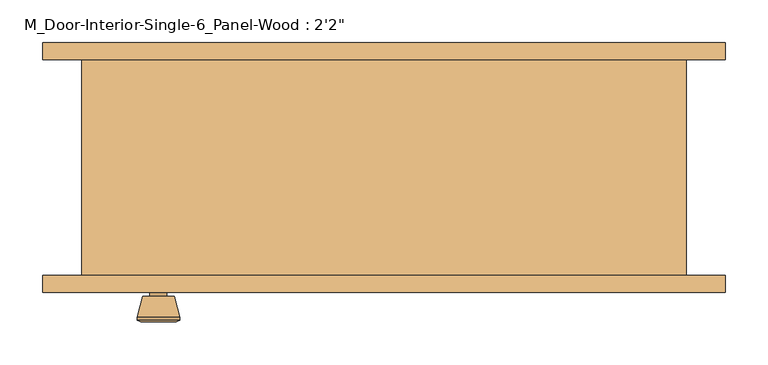
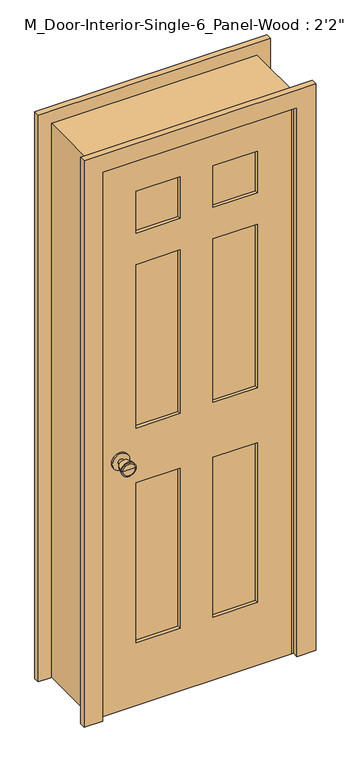
"""IFC4 building model written with IfcOpenShell, lengths in millimetres: door geometry."""

from ifc_helpers import new_model, si_unit, point, frame, frame_2d, origin, place, context, project, spatial, polyline, circle_curve, trimmed, segment, composite_curve, outline, extrude, faceted_brep, source, transform, mapped, element, save
from ifc_brep_helpers import plane_surface, cylinder_surface, revolved_surface, advanced_brep


def door_809e0d7a(model_context):
    return source(origin(), model_context, "Body", "SolidModel", [
        advanced_brep(
        [(-265.2, -82.825, 914.4), (-275.2, -82.825, 914.4), (-255.2, -82.825, 914.4), (-244.7241324, -33.825, 914.4), (-285.6758676, -33.825, 914.4), (-265.2, -33.825, 914.4), (-240.2, -35.6528681, 914.4), (-290.2, -35.6528681, 914.4), (-240.2, -39.1165463, 914.4), (-290.2, -39.1165463, 914.4), (-246.563764, -63.825, 914.4), (-283.836236, -63.825, 914.4), (-255.2, -63.825, 914.4), (-275.2, -63.825, 914.4)],
        [
            (0, 1),
            (1, 2, circle_curve(frame((-265.2, -82.825, 914.4), z_axis=(0.0, -1.0, 0.0), x_axis=(-1.0, 0.0, 0.0)), 10.0)),
            (2, 0),
            (2, 1, circle_curve(frame((-265.2, -82.825, 914.4), z_axis=(0.0, -1.0, 0.0), x_axis=(-1.0, 0.0, 0.0)), 10.0)),
            (3, 4, circle_curve(frame((-265.2, -33.825, 914.4), z_axis=(0.0, 1.0, 0.0), x_axis=(-1.0, 0.0, 0.0)), 20.4758676)),
            (4, 5),
            (5, 3),
            (4, 3, circle_curve(frame((-265.2, -33.825, 914.4), z_axis=(0.0, 1.0, 0.0), x_axis=(-1.0, 0.0, 0.0)), 20.4758676)),
            (6, 7, circle_curve(frame((-265.2, -35.6528681, 914.4), z_axis=(0.0, 1.0, 0.0), x_axis=(-1.0, 0.0, 0.0)), 25.0)),
            (7, 4),
            (3, 6),
            (7, 6, circle_curve(frame((-265.2, -35.6528681, 914.4), z_axis=(0.0, 1.0, 0.0), x_axis=(-1.0, 0.0, 0.0)), 25.0)),
            (8, 9, circle_curve(frame((-265.2, -39.1165463, 914.4), z_axis=(0.0, 1.0, 0.0), x_axis=(-1.0, 0.0, 0.0)), 25.0)),
            (9, 7),
            (6, 8),
            (9, 8, circle_curve(frame((-265.2, -39.1165463, 914.4), z_axis=(0.0, 1.0, 0.0), x_axis=(-1.0, 0.0, 0.0)), 25.0)),
            (10, 11, circle_curve(frame((-265.2, -63.825, 914.4), z_axis=(0.0, 1.0, 0.0), x_axis=(-1.0, 0.0, 0.0)), 18.636236)),
            (11, 9),
            (8, 10),
            (11, 10, circle_curve(frame((-265.2, -63.825, 914.4), z_axis=(0.0, 1.0, 0.0), x_axis=(-1.0, 0.0, 0.0)), 18.636236)),
            (12, 13, circle_curve(frame((-265.2, -63.825, 914.4), z_axis=(0.0, 1.0, 0.0), x_axis=(-1.0, 0.0, 0.0)), 10.0)),
            (13, 11),
            (10, 12),
            (13, 12, circle_curve(frame((-265.2, -63.825, 914.4), z_axis=(0.0, 1.0, 0.0), x_axis=(-1.0, 0.0, 0.0)), 10.0)),
            (1, 13),
            (12, 2),
        ],
        [
            plane_surface(frame((-265.2, -82.825, 914.4), z_axis=(0.0, -1.0, 0.0), x_axis=(-1.0, 0.0, 0.0))),
            plane_surface(frame((-265.2, -33.825, 914.4), z_axis=(0.0, 1.0, 0.0), x_axis=(-1.0, 0.0, 0.0))),
            revolved_surface(polyline([(-285.6758676, -33.825, 914.4), (-290.2, -35.6528681, 914.4)]), (-265.2, -82.825, 914.4), (0.0, -1.0, 0.0)),
            cylinder_surface(frame((-265.2, -82.825, 914.4), z_axis=(0.0, -1.0, 0.0), x_axis=(-1.0, 0.0, 0.0)), 25.0),
            revolved_surface(polyline([(-290.2, -39.1165463, 914.4), (-283.836236, -63.825, 914.4)]), (-265.2, -82.825, 914.4), (0.0, -1.0, 0.0)),
            plane_surface(frame((-265.2, -63.825, 914.4), z_axis=(0.0, -1.0, 0.0), x_axis=(-1.0, 0.0, 0.0))),
            cylinder_surface(frame((-265.2, -82.825, 914.4), z_axis=(0.0, -1.0, 0.0), x_axis=(-1.0, 0.0, 0.0)), 10.0),
        ],
        [
            (0, [[1, 2, 3]]),
            (0, [[-3, 4, -1]]),
            (1, [[5, 6, 7]]),
            (1, [[8, -7, -6]]),
            (2, [[9, 10, -5, 11]]),
            (2, [[12, -11, -8, -10]]),
            (3, [[13, 14, -9, 15]]),
            (3, [[16, -15, -12, -14]]),
            (4, [[17, 18, -13, 19]]),
            (4, [[20, -19, -16, -18]]),
            (5, [[21, 22, -17, 23]]),
            (5, [[24, -23, -20, -22]]),
            (6, [[-2, 25, -21, 26]]),
            (6, [[-4, -26, -24, -25]]),
        ],
    ),
        extrude(outline(composite_curve([segment(trimmed(circle_curve(frame_2d((914.4, -265.2)), 30.0), [point((914.4, -295.2))], [point((914.4, -235.2))], False, "CARTESIAN"), True, "CONTINUOUS"), segment(trimmed(circle_curve(frame_2d((914.4, -265.2)), 30.0), [point((914.4, -235.2))], [point((914.4, -295.2))], False, "CARTESIAN"), True, "CONTINUOUS")], self_intersect=False)), frame((0.0, -88.825, 0.0), z_axis=(0.0, 1.0, 0.0), x_axis=(0.0, 0.0, 1.0)), (0.0, 0.0, 1.0), 6.0),
        advanced_brep(
        [(-265.2, -129.825, 914.4), (-255.2, -129.825, 914.4), (-275.2, -129.825, 914.4), (-244.7241324, -178.825, 914.4), (-265.2, -178.825, 914.4), (-285.6758676, -178.825, 914.4), (-240.2, -176.9971319, 914.4), (-290.2, -176.9971319, 914.4), (-240.2, -173.5334537, 914.4), (-290.2, -173.5334537, 914.4), (-246.563764, -148.825, 914.4), (-283.836236, -148.825, 914.4), (-255.2, -148.825, 914.4), (-275.2, -148.825, 914.4)],
        [
            (0, 1),
            (1, 2, circle_curve(frame((-265.2, -129.825, 914.4), z_axis=(0.0, 1.0, 0.0), x_axis=(-1.0, 0.0, 0.0)), 10.0)),
            (2, 0),
            (2, 1, circle_curve(frame((-265.2, -129.825, 914.4), z_axis=(0.0, 1.0, 0.0), x_axis=(-1.0, 0.0, 0.0)), 10.0)),
            (3, 4),
            (4, 5),
            (5, 3, circle_curve(frame((-265.2, -178.825, 914.4), z_axis=(0.0, -1.0, 0.0), x_axis=(-1.0, 0.0, 0.0)), 20.4758676)),
            (3, 5, circle_curve(frame((-265.2, -178.825, 914.4), z_axis=(0.0, -1.0, 0.0), x_axis=(-1.0, 0.0, 0.0)), 20.4758676)),
            (6, 3),
            (5, 7),
            (7, 6, circle_curve(frame((-265.2, -176.9971319, 914.4), z_axis=(0.0, -1.0, 0.0), x_axis=(-1.0, 0.0, 0.0)), 25.0)),
            (6, 7, circle_curve(frame((-265.2, -176.9971319, 914.4), z_axis=(0.0, -1.0, 0.0), x_axis=(-1.0, 0.0, 0.0)), 25.0)),
            (8, 6),
            (7, 9),
            (9, 8, circle_curve(frame((-265.2, -173.5334537, 914.4), z_axis=(0.0, -1.0, 0.0), x_axis=(-1.0, 0.0, 0.0)), 25.0)),
            (8, 9, circle_curve(frame((-265.2, -173.5334537, 914.4), z_axis=(0.0, -1.0, 0.0), x_axis=(-1.0, 0.0, 0.0)), 25.0)),
            (10, 8),
            (9, 11),
            (11, 10, circle_curve(frame((-265.2, -148.825, 914.4), z_axis=(0.0, -1.0, 0.0), x_axis=(-1.0, 0.0, 0.0)), 18.636236)),
            (10, 11, circle_curve(frame((-265.2, -148.825, 914.4), z_axis=(0.0, -1.0, 0.0), x_axis=(-1.0, 0.0, 0.0)), 18.636236)),
            (12, 10),
            (11, 13),
            (13, 12, circle_curve(frame((-265.2, -148.825, 914.4), z_axis=(0.0, -1.0, 0.0), x_axis=(-1.0, 0.0, 0.0)), 10.0)),
            (12, 13, circle_curve(frame((-265.2, -148.825, 914.4), z_axis=(0.0, -1.0, 0.0), x_axis=(-1.0, 0.0, 0.0)), 10.0)),
            (1, 12),
            (13, 2),
        ],
        [
            plane_surface(frame((-265.2, -129.825, 914.4), z_axis=(0.0, 1.0, 0.0), x_axis=(-1.0, 0.0, 0.0))),
            plane_surface(frame((-265.2, -178.825, 914.4), z_axis=(0.0, -1.0, 0.0), x_axis=(-1.0, 0.0, 0.0))),
            revolved_surface(polyline([(-285.6758676, -178.825, 914.4), (-290.2, -176.9971319, 914.4)]), (-265.2, -129.825, 914.4), (0.0, 1.0, 0.0)),
            cylinder_surface(frame((-265.2, -129.825, 914.4), z_axis=(0.0, 1.0, 0.0), x_axis=(-1.0, 0.0, 0.0)), 25.0),
            revolved_surface(polyline([(-290.2, -173.5334537, 914.4), (-283.836236, -148.825, 914.4)]), (-265.2, -129.825, 914.4), (0.0, 1.0, 0.0)),
            plane_surface(frame((-265.2, -148.825, 914.4), z_axis=(0.0, 1.0, 0.0), x_axis=(-1.0, 0.0, 0.0))),
            cylinder_surface(frame((-265.2, -129.825, 914.4), z_axis=(0.0, 1.0, 0.0), x_axis=(-1.0, 0.0, 0.0)), 10.0),
        ],
        [
            (0, [[1, 2, 3]]),
            (0, [[-3, 4, -1]]),
            (1, [[5, 6, 7]]),
            (1, [[-6, -5, 8]]),
            (2, [[9, -7, 10, 11]]),
            (2, [[-10, -8, -9, 12]]),
            (3, [[13, -11, 14, 15]]),
            (3, [[-14, -12, -13, 16]]),
            (4, [[17, -15, 18, 19]]),
            (4, [[-18, -16, -17, 20]]),
            (5, [[21, -19, 22, 23]]),
            (5, [[-22, -20, -21, 24]]),
            (6, [[25, -23, 26, -2]]),
            (6, [[-26, -24, -25, -4]]),
        ],
    ),
        extrude(outline(composite_curve([segment(trimmed(circle_curve(frame_2d((914.4, -265.2)), 30.0), [point((914.4, -295.2))], [point((914.4, -235.2))], False, "CARTESIAN"), True, "CONTINUOUS"), segment(trimmed(circle_curve(frame_2d((914.4, -265.2)), 30.0), [point((914.4, -235.2))], [point((914.4, -295.2))], False, "CARTESIAN"), True, "CONTINUOUS")], self_intersect=False)), frame((0.0, -129.825, 0.0), z_axis=(0.0, 1.0, 0.0), x_axis=(0.0, 0.0, 1.0)), (0.0, 0.0, 1.0), 6.0),
        faceted_brep([(355.2, -123.825, 0.0), (330.2, -123.825, 0.0), (330.2, -88.825, 0.0), (317.5, -88.825, 0.0), (317.5, -53.9, 0.0), (330.2, -53.9, 0.0), (330.2, 130.175, 0.0), (355.2, 130.175, 0.0), (355.2, 130.175, 2025.0), (355.2, -123.825, 2025.0), (330.2, 130.175, 2000.0), (-330.2, 130.175, 2000.0), (-330.2, 130.175, 0.0), (-355.2, 130.175, 0.0), (-355.2, 130.175, 2025.0), (330.2, -53.9, 2000.0), (317.5, -53.9, 1987.3), (-317.5, -53.9, 1987.3), (-317.5, -53.9, 0.0), (-330.2, -53.9, 0.0), (-330.2, -53.9, 2000.0), (317.5, -88.825, 1987.3), (330.2, -88.825, 2000.0), (-330.2, -88.825, 2000.0), (-330.2, -88.825, 0.0), (-317.5, -88.825, 0.0), (-317.5, -88.825, 1987.3), (330.2, -123.825, 2000.0), (-355.2, -123.825, 2025.0), (-355.2, -123.825, 0.0), (-330.2, -123.825, 0.0), (-330.2, -123.825, 2000.0)], [[[0, 1, 2, 3, 4, 5, 6, 7]], [[7, 8, 9, 0]], [[6, 10, 11, 12, 13, 14, 8, 7]], [[5, 15, 10, 6]], [[4, 16, 17, 18, 19, 20, 15, 5]], [[3, 21, 16, 4]], [[2, 22, 23, 24, 25, 26, 21, 3]], [[1, 27, 22, 2]], [[0, 9, 28, 29, 30, 31, 27, 1]], [[8, 14, 28, 9]], [[15, 20, 11, 10]], [[21, 26, 17, 16]], [[27, 31, 23, 22]], [[29, 13, 12, 19, 18, 25, 24, 30]], [[14, 13, 29, 28]], [[20, 19, 12, 11]], [[26, 25, 18, 17]], [[31, 30, 24, 23]]]),
        extrude(outline(polyline([(2000.0, -330.2), (0.0, -330.2), (0.0, 330.2), (2000.0, 330.2), (2000.0, -330.2)]), holes=[polyline([(1880.0, 57.5), (1880.0, 210.2), (1727.3, 210.2), (1727.3, 57.5), (1880.0, 57.5)]), polyline([(1612.3, 210.2), (1014.4, 210.2), (1014.4, 57.5), (1612.3, 57.5), (1612.3, 210.2)]), polyline([(1014.4, -57.5), (1014.4, -210.2), (1612.3, -210.2), (1612.3, -57.5), (1014.4, -57.5)]), polyline([(1727.3, -210.2), (1880.0, -210.2), (1880.0, -57.5), (1727.3, -57.5), (1727.3, -210.2)]), polyline([(814.4, 57.5), (814.4, 210.2), (230.0, 210.2), (230.0, 57.5), (814.4, 57.5)]), polyline([(230.0, -57.5), (230.0, -210.2), (814.4, -210.2), (814.4, -57.5), (230.0, -57.5)])]), frame((0.0, -123.825, 0.0), z_axis=(0.0, 1.0, 0.0), x_axis=(0.0, 0.0, 1.0)), (0.0, 0.0, 1.0), 35.0),
        extrude(outline(polyline([(210.2, -100.4916667), (210.2, -112.1583333), (57.5, -112.1583333), (57.5, -100.4916667), (210.2, -100.4916667)])), frame((0.0, 0.0, 1727.3), z_axis=(0.0, 0.0, 1.0), x_axis=(1.0, 0.0, 0.0)), (0.0, 0.0, 1.0), 152.7),
        extrude(outline(polyline([(210.2, -100.4916667), (210.2, -112.1583333), (57.5, -112.1583333), (57.5, -100.4916667), (210.2, -100.4916667)])), frame((0.0, 0.0, 1014.4), z_axis=(0.0, 0.0, 1.0), x_axis=(1.0, 0.0, 0.0)), (0.0, 0.0, 1.0), 597.9),
        extrude(outline(polyline([(-57.5, -100.4916667), (-57.5, -112.1583333), (-210.2, -112.1583333), (-210.2, -100.4916667), (-57.5, -100.4916667)])), frame((0.0, 0.0, 1014.4), z_axis=(0.0, 0.0, 1.0), x_axis=(1.0, 0.0, 0.0)), (0.0, 0.0, 1.0), 597.9),
        extrude(outline(polyline([(-57.5, -100.4916667), (-57.5, -112.1583333), (-210.2, -112.1583333), (-210.2, -100.4916667), (-57.5, -100.4916667)])), frame((0.0, 0.0, 1727.3), z_axis=(0.0, 0.0, 1.0), x_axis=(1.0, 0.0, 0.0)), (0.0, 0.0, 1.0), 152.7),
        extrude(outline(polyline([(210.2, -100.4916667), (210.2, -112.1583333), (57.5, -112.1583333), (57.5, -100.4916667), (210.2, -100.4916667)])), frame((0.0, 0.0, 230.0), z_axis=(0.0, 0.0, 1.0), x_axis=(1.0, 0.0, 0.0)), (0.0, 0.0, 1.0), 584.4),
        extrude(outline(polyline([(-57.5, -100.4916667), (-57.5, -112.1583333), (-210.2, -112.1583333), (-210.2, -100.4916667), (-57.5, -100.4916667)])), frame((0.0, 0.0, 230.0), z_axis=(0.0, 0.0, 1.0), x_axis=(1.0, 0.0, 0.0)), (0.0, 0.0, 1.0), 584.4),
        extrude(outline(polyline([(0.0, 401.55), (2071.35, 401.55), (2071.35, -401.55), (0.0, -401.55), (0.0, -336.55), (2006.35, -336.55), (2006.35, 336.55), (0.0, 336.55), (0.0, 401.55)])), frame((0.0, -143.825, 0.0), z_axis=(0.0, 1.0, 0.0), x_axis=(0.0, 0.0, 1.0)), (0.0, 0.0, 1.0), 20.0),
        extrude(outline(polyline([(0.0, 401.55), (2071.35, 401.55), (2071.35, -401.55), (0.0, -401.55), (0.0, -336.55), (2006.35, -336.55), (2006.35, 336.55), (0.0, 336.55), (0.0, 401.55)])), frame((0.0, 130.175, 0.0), z_axis=(0.0, 1.0, 0.0), x_axis=(0.0, 0.0, 1.0)), (0.0, 0.0, 1.0), 20.0),
    ])


if __name__ == "__main__":
    model = new_model("IFC4")
    model_context = context("Model", 3, world=origin())
    ifc_project = project(units=[si_unit("LENGTHUNIT", "METRE", prefix="MILLI")], contexts=[model_context])
    site = spatial("IfcSite", under=ifc_project)
    building = spatial("IfcBuilding", under=site)
    placement = place(None, origin())
    door_shape = door_809e0d7a(model_context)
    element("IfcDoor", 1, ObjectType="M_Door-Interior-Single-6_Panel-Wood : 2'2\"", at=placement, inside=building, context=model_context, shape_type="MappedRepresentation", body=[
        mapped(door_shape, transform((0.0, 0.0, 0.0), x_axis=(1.0, 0.0, 0.0), y_axis=(0.0, 1.0, 0.0), z_axis=(0.0, 0.0, 1.0))),
    ])
    save(model, "model.ifc")

# Revit data of these elements
# Type "M_Door-Interior-Single-6_Panel-Wood : 2'2\""
#   Type Mark = "47"
#   Assembly Code = "C1020300"
#   Analytic Construction = "Wooden"
#   Top Rail = 0' - 4.72441"
#   Top Panel = 0' - 6.01181"
#   Thickness = 0' - 1.37795"
#   Thermal Resistance (R) = 0.455703 (m²·K)/W
#   Swing Angle [instance default] = 90.00°
#   Stiles = 0' - 4.72441"
#   Rough Width = 2' - 3.9685"
#   Rough Height = 6' - 7.72441"
#   Mullion = 0' - 4.52756"
#   Lock Rail = 0' - 7.87402"
#   Intermediate Rail = 0' - 4.52756"
#   Height = 6' - 6.74016"
#   Width = 2' - 2"
#   Heat Transfer Coefficient (U) = 2.19465 W/(m²·K)
#   Bottom Rail = 0' - 9.05512"
#   Trim Material = Cherry
#   Panel Material = Cherry
#   Frame Material = Cherry
#   Door Handle Material = Aluminum
#   Visual Light Transmittance = 0
#   Solar Heat Gain Coefficient = 0
#   Wall Closure = (empty or 0)
#   Function = (empty or 0)
# Element 1 (IfcDoor, "M_Door-Interior-Single-6_Panel-Wood : 2'2\"")
#   Materials on its faces: "Cherry", "Aluminum"
# Materials
#   "Cherry": class "Wood", colour RGB 226 177 128, transparency 0, Description = "Prunus Serotina", Cost = 0
#   "Aluminum": class "Metal", colour RGB 247 247 247, transparency 0, Description = "Aluminum 6061", Cost = 0
